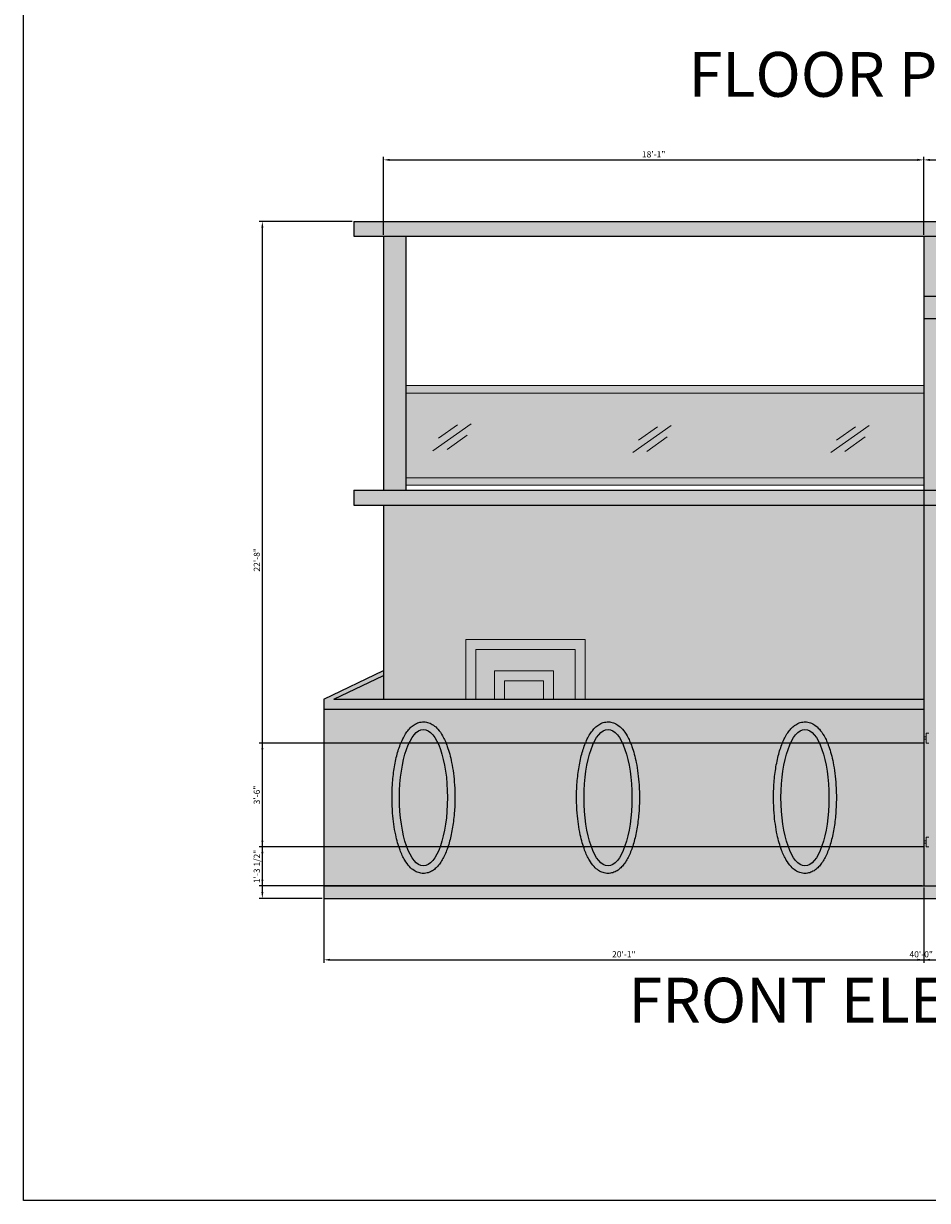
# Model space of a CAD drawing. Units: inches. Extents: x 2169 to 10664, y 1669 to 6352.
# Tile 13 of 17: x 9415 to 9778, y 5159 to 5632. Entities that reach past the tile are written whole.
import ezdxf

# ---------------------------------------------------------------- set-up
doc = ezdxf.new("R2010")
doc.units = ezdxf.units.IN
for name, color, linetype, lineweight in [('A-ANNO-DIMS', 3, 'Continuous', 18), ('A-ANNO-TITL', 3, 'Continuous', 25), ('A-ANNO-TTLB', 7, 'Continuous', 25), ('A-ELEV', 7, 'Continuous', 25), ('A-ELEV-CONC-PATT', 85, 'Continuous', 13), ('A-ELEV-GATE', 7, 'Continuous', 18), ('A-ELEV-GATE-PATT', 252, 'Continuous', 13), ('A-ELEV-OPEN', 7, 'Continuous', 18), ('A-ELEV-OPEN-PATT', 9, 'Continuous', 13), ('A-ELEV-PATT', 253, 'Continuous', 13)]:
    doc.layers.add(name, color=color, linetype=linetype, lineweight=lineweight)
doc.styles.get("Standard").update_dxf_attribs({"font": 'arial.ttf'})
doc.dimstyles.new('ISO-25', dxfattribs={"dimtxt": 2.5, "dimasz": 2.5, "dimexe": 1.25, "dimexo": 0.625, "dimtad": 1, "dimdec": 0, "dimlunit": 3, "dimtxsty": 'Standard', "dimcen": 2.5, "dimadec": 0, "dimazin": 0, "dimtfac": 1, "dimtdec": 0, "dimtmove": 0, "dimatfit": 3, "dimfxl": 1, "dimarcsym": 0})

# ---------------------------------------------------------------- blocks, each defined once
blk = doc.blocks.new('GLASS-MARK-B')
for p, q in [((0, 0), (15.39, 10.84)), ((2.27, 5.02), (9.88, 10.35)), ((5.67, 0.49), (13.77, 6.31))]:
    blk.add_line(p, q)
blk = doc.blocks.new('GATE-HINGE-3')
for p, q in [((1, 2.5), (0, 2.5)), ((1, 1.5), (0, 1.5)), ((2, 4), (1, 4)), ((1, 4), (1, 0)), ((2, 0), (1, 0))]:
    blk.add_line(p, q)
blk = doc.blocks.new('FACADE-OVAL-INSET')
blk.add_ellipse((12.63, 30.44), major_axis=(0, -27.44), ratio=0.350877)
blk.add_open_spline([(12.63, 0), (13.28, 0), (13.93, 0.1), (15.16, 0.48), (15.73, 0.75), (16.8, 1.42), (17.29, 1.81), (18.2, 2.68), (18.63, 3.16), (19.86, 4.78), (20.59, 6.05), (21.9, 8.93), (22.47, 10.53), (23.47, 14), (23.89, 15.87), (24.57, 19.81), (24.82, 21.88), (25.3, 27.78), (25.34, 31.73), (24.89, 38.68), (24.51, 41.73), (23.49, 46.87), (22.91, 49.03), (21.66, 52.55), (21.03, 53.98), (19.74, 56.25), (19.12, 57.16), (17.87, 58.57), (17.27, 59.12), (16.05, 59.96), (15.45, 60.28), (14.17, 60.73), (13.48, 60.86), (12.09, 60.9), (11.4, 60.8), (10.08, 60.4), (9.47, 60.11), (8.34, 59.39), (7.83, 58.96), (6.87, 58.01), (6.43, 57.49), (5.17, 55.76), (4.44, 54.41), (3.14, 51.39), (2.57, 49.71), (1.59, 46.07), (1.19, 44.12), (0.55, 40.02), (0.31, 37.87), (-0.08, 31.9), (-0.06, 28), (0.48, 21.2), (0.89, 18.26), (1.95, 13.31), (2.54, 11.23), (3.8, 7.86), (4.43, 6.5), (5.71, 4.33), (6.34, 3.47), (7.58, 2.13), (8.18, 1.61), (9.39, 0.82), (9.99, 0.52), (11.27, 0.11), (11.95, 0), (12.63, 0)], degree=3, knots=[0, 0, 0, 0, 0.107478, 0.107478, 0.214955, 0.214955, 0.322433, 0.322433, 0.429911, 0.429911, 0.658113, 0.658113, 0.886316, 0.886316, 1.114519, 1.114519, 1.342721, 1.342721, 1.750863, 1.750863, 2.0857, 2.0857, 2.362812, 2.362812, 2.586848, 2.586848, 2.764909, 2.764909, 2.903641, 2.903641, 3.018249, 3.018249, 3.132858, 3.132858, 3.247466, 3.247466, 3.362074, 3.362074, 3.476683, 3.476683, 3.591291, 3.591291, 3.82536, 3.82536, 4.059428, 4.059428, 4.293497, 4.293497, 4.527566, 4.527566, 4.931556, 4.931556, 5.258929, 5.258929, 5.530471, 5.530471, 5.749212, 5.749212, 5.922827, 5.922827, 6.058126, 6.058126, 6.171203, 6.171203, 6.283185, 6.283185, 6.283185, 6.283185])
blk = doc.blocks.new('*D117')
at = {"layer": 'A-ANNO-DIMS', "color": 0, "lineweight": -2, "transparency": 16777216}
for p, q in [((9535.46, 5279.69), (9535.46, 5254.36)), ((10015.46, 5279.69), (10015.46, 5254.36)), ((9537.96, 5255.61), (10012.96, 5255.61))]:
    blk.add_line(p, q, dxfattribs=at)
at = {"layer": 'A-ANNO-DIMS', "color": 0, "transparency": 16777216}
for points in [[(9537.96, 5256.03), (9537.96, 5255.19), (9535.46, 5255.61)], [(10012.96, 5256.03), (10012.96, 5255.19), (10015.46, 5255.61)]]:
    blk.add_solid(points, dxfattribs=at)
at = {"layer": 'Defpoints', "color": 0, "transparency": 16777216}
for p in [(9535.46, 5280.31), (10015.46, 5280.31), (10015.46, 5255.61)]:
    blk.add_point(p, dxfattribs=at)
at = {"layer": 'A-ANNO-DIMS', "color": 0, "transparency": 16777216, "insert": (9775.46, 5257.51), "char_height": 2.5, "attachment_point": 5}
blk.add_mtext('40\'-0"', dxfattribs=at)
blk = doc.blocks.new('*D118')
at = {"layer": 'A-ANNO-DIMS', "color": 0, "lineweight": -2, "transparency": 16777216}
for p, q in [((9546.84, 5552.31), (9509.51, 5552.31)), ((9510.76, 5282.81), (9510.76, 5549.81)), ((9534.84, 5280.31), (9509.51, 5280.31))]:
    blk.add_line(p, q, dxfattribs=at)
at = {"layer": 'A-ANNO-DIMS', "color": 0, "transparency": 16777216}
for points in [[(9510.35, 5549.81), (9511.18, 5549.81), (9510.76, 5552.31)], [(9510.35, 5282.81), (9511.18, 5282.81), (9510.76, 5280.31)]]:
    blk.add_solid(points, dxfattribs=at)
at = {"layer": 'Defpoints', "color": 0, "transparency": 16777216}
for p in [(9510.76, 5552.31), (9547.46, 5552.31), (9535.46, 5280.31)]:
    blk.add_point(p, dxfattribs=at)
at = {"layer": 'A-ANNO-DIMS', "color": 0, "transparency": 16777216, "insert": (9508.86, 5416.31), "char_height": 2.5, "attachment_point": 5, "rotation": 90}
blk.add_mtext('22\'-8"', dxfattribs=at)
blk = doc.blocks.new('*D120')
at = {"layer": 'A-ANNO-DIMS', "color": 0, "lineweight": -2, "transparency": 16777216}
for p, q in [((9535.46, 5284.69), (9535.46, 5254.36)), ((9776.46, 5284.69), (9776.46, 5254.36)), ((9537.96, 5255.61), (9773.96, 5255.61))]:
    blk.add_line(p, q, dxfattribs=at)
at = {"layer": 'A-ANNO-DIMS', "color": 0, "transparency": 16777216}
for points in [[(9537.96, 5256.03), (9537.96, 5255.19), (9535.46, 5255.61)], [(9773.96, 5256.03), (9773.96, 5255.19), (9776.46, 5255.61)]]:
    blk.add_solid(points, dxfattribs=at)
at = {"layer": 'Defpoints', "color": 0, "transparency": 16777216}
for p in [(9535.46, 5285.31), (9776.46, 5285.31), (9776.46, 5255.61)]:
    blk.add_point(p, dxfattribs=at)
at = {"layer": 'A-ANNO-DIMS', "color": 0, "transparency": 16777216, "insert": (9655.96, 5257.51), "char_height": 2.5, "attachment_point": 5}
blk.add_mtext('20\'-1"', dxfattribs=at)
blk = doc.blocks.new('*D121')
at = {"layer": 'A-ANNO-DIMS', "color": 0, "lineweight": -2, "transparency": 16777216}
for p, q in [((9559.46, 5546.94), (9559.46, 5578.26)), ((9561.96, 5577.01), (9773.96, 5577.01)), ((9776.46, 5546.94), (9776.46, 5578.26))]:
    blk.add_line(p, q, dxfattribs=at)
at = {"layer": 'A-ANNO-DIMS', "color": 0, "transparency": 16777216}
for points in [[(9561.96, 5577.43), (9561.96, 5576.59), (9559.46, 5577.01)], [(9773.96, 5577.43), (9773.96, 5576.59), (9776.46, 5577.01)]]:
    blk.add_solid(points, dxfattribs=at)
at = {"layer": 'Defpoints', "color": 0, "transparency": 16777216}
for p in [(9776.46, 5577.01), (9559.46, 5546.31), (9776.46, 5546.31)]:
    blk.add_point(p, dxfattribs=at)
at = {"layer": 'A-ANNO-DIMS', "color": 0, "transparency": 16777216, "insert": (9667.96, 5578.91), "char_height": 2.5, "attachment_point": 5}
blk.add_mtext('18\'-1"', dxfattribs=at)
blk = doc.blocks.new('*D122')
at = {"layer": 'A-ANNO-DIMS', "color": 0, "lineweight": -2, "transparency": 16777216}
for p, q in [((9776.46, 5546.94), (9776.46, 5578.26)), ((9778.96, 5577.01), (9932.96, 5577.01)), ((9935.46, 5546.94), (9935.46, 5578.26))]:
    blk.add_line(p, q, dxfattribs=at)
at = {"layer": 'A-ANNO-DIMS', "color": 0, "transparency": 16777216}
for points in [[(9778.96, 5577.43), (9778.96, 5576.59), (9776.46, 5577.01)], [(9932.96, 5577.43), (9932.96, 5576.59), (9935.46, 5577.01)]]:
    blk.add_solid(points, dxfattribs=at)
at = {"layer": 'Defpoints', "color": 0, "transparency": 16777216}
for p in [(9935.46, 5577.01), (9776.46, 5546.31), (9935.46, 5546.31)]:
    blk.add_point(p, dxfattribs=at)
at = {"layer": 'A-ANNO-DIMS', "color": 0, "transparency": 16777216, "insert": (9855.96, 5578.91), "char_height": 2.5, "attachment_point": 5}
blk.add_mtext('13\'-3"', dxfattribs=at)
blk = doc.blocks.new('*D124')
at = {"layer": 'A-ANNO-DIMS', "color": 0, "lineweight": -2, "transparency": 16777216}
for p, q in [((9776.46, 5284.69), (9776.46, 5254.36)), ((9848.46, 5284.69), (9848.46, 5254.36)), ((9778.96, 5255.61), (9845.96, 5255.61))]:
    blk.add_line(p, q, dxfattribs=at)
at = {"layer": 'A-ANNO-DIMS', "color": 0, "transparency": 16777216}
for points in [[(9778.96, 5256.03), (9778.96, 5255.19), (9776.46, 5255.61)], [(9845.96, 5256.03), (9845.96, 5255.19), (9848.46, 5255.61)]]:
    blk.add_solid(points, dxfattribs=at)
at = {"layer": 'Defpoints', "color": 0, "transparency": 16777216}
for p in [(9776.46, 5285.31), (9848.46, 5285.31), (9848.46, 5255.61)]:
    blk.add_point(p, dxfattribs=at)
at = {"layer": 'A-ANNO-DIMS', "color": 0, "transparency": 16777216, "insert": (9812.46, 5257.51), "char_height": 2.5, "attachment_point": 5}
blk.add_mtext('6\'-0"', dxfattribs=at)
blk = doc.blocks.new('*D126')
at = {"layer": 'A-ANNO-DIMS', "color": 0, "lineweight": -2, "transparency": 16777216}
for p, q in [((9776.84, 5300.95), (9509.51, 5300.95)), ((9510.76, 5287.81), (9510.76, 5298.45)), ((9775.84, 5285.31), (9509.51, 5285.31))]:
    blk.add_line(p, q, dxfattribs=at)
at = {"layer": 'A-ANNO-DIMS', "color": 0, "transparency": 16777216}
for points in [[(9510.35, 5298.45), (9511.18, 5298.45), (9510.76, 5300.95)], [(9510.35, 5287.81), (9511.18, 5287.81), (9510.76, 5285.31)]]:
    blk.add_solid(points, dxfattribs=at)
at = {"layer": 'Defpoints', "color": 0, "transparency": 16777216}
for p in [(9510.76, 5300.95), (9777.46, 5300.95), (9776.46, 5285.31)]:
    blk.add_point(p, dxfattribs=at)
at = {"layer": 'A-ANNO-DIMS', "color": 0, "transparency": 16777216, "insert": (9508.84, 5293.13), "char_height": 2.5, "attachment_point": 5, "rotation": 90}
blk.add_mtext('1\'-3 1/2"', dxfattribs=at)
blk = doc.blocks.new('*D127')
at = {"layer": 'A-ANNO-DIMS', "color": 0, "lineweight": -2, "transparency": 16777216}
for p, q in [((9776.84, 5342.71), (9509.51, 5342.71)), ((9510.76, 5303.45), (9510.76, 5340.21)), ((9776.84, 5300.95), (9509.51, 5300.95))]:
    blk.add_line(p, q, dxfattribs=at)
at = {"layer": 'A-ANNO-DIMS', "color": 0, "transparency": 16777216}
for points in [[(9510.35, 5340.21), (9511.18, 5340.21), (9510.76, 5342.71)], [(9510.35, 5303.45), (9511.18, 5303.45), (9510.76, 5300.95)]]:
    blk.add_solid(points, dxfattribs=at)
at = {"layer": 'Defpoints', "color": 0, "transparency": 16777216}
for p in [(9510.76, 5342.71), (9777.46, 5342.71), (9777.46, 5300.95)]:
    blk.add_point(p, dxfattribs=at)
at = {"layer": 'A-ANNO-DIMS', "color": 0, "transparency": 16777216, "insert": (9508.86, 5321.83), "char_height": 2.5, "attachment_point": 5, "rotation": 90}
blk.add_mtext('3\'-6"', dxfattribs=at)

msp = doc.modelspace()

# ---------------------------------------------------------------- hatches: boundary and pattern name
at = {"layer": 'A-ELEV-CONC-PATT'}
h = msp.add_hatch(dxfattribs=at)
h.set_pattern_fill('AR-CONC', color=256, scale=0.02)
h.paths.add_polyline_path([(9899.46, 5522.31), (9776.46, 5522.31), (9776.46, 5513.31), (9890.46, 5513.31), (9890.46, 5444.31), (9899.46, 5444.31)])
h.paths.add_polyline_path([(9899.46, 5438.31), (9890.46, 5438.31), (9890.46, 5285.31), (9899.46, 5285.31)])
at = {"layer": 'A-ELEV-GATE-PATT'}
h = msp.add_hatch(color=256, dxfattribs=at)
h.dxf.hatch_style = 1
h.paths.add_polyline_path([(9778.46, 5346.71), (9777.46, 5346.71), (9777.46, 5342.71), (9778.46, 5342.71)])
h.paths.add_polyline_path([(9777.46, 5345.21), (9776.46, 5345.21), (9776.46, 5344.21), (9777.46, 5344.21)])
h.paths.add_polyline_path([(9848.46, 5345.21), (9847.46, 5345.21), (9847.46, 5344.21), (9848.46, 5344.21)])
h.paths.add_polyline_path([(9847.46, 5346.71), (9846.46, 5346.71), (9846.46, 5342.71), (9847.46, 5342.71)])
h.paths.add_polyline_path([(9847.46, 5304.95), (9846.46, 5304.95), (9846.46, 5300.95), (9847.46, 5300.95)])
h.paths.add_polyline_path([(9848.46, 5303.45), (9847.46, 5303.45), (9847.46, 5302.45), (9848.46, 5302.45)])
h.paths.add_polyline_path([(9778.46, 5304.95), (9777.46, 5304.95), (9777.46, 5300.95), (9778.46, 5300.95)])
h.paths.add_polyline_path([(9777.46, 5303.45), (9776.46, 5303.45), (9776.46, 5302.45), (9777.46, 5302.45)])
h.paths.add_polyline_path([(9811.96, 5360.31), (9778.46, 5360.31), (9778.46, 5287.31), (9811.96, 5287.31)])
h.paths.add_polyline_path([(9783.46, 5355.31), (9806.96, 5355.31), (9806.96, 5292.31), (9783.46, 5292.31)], flags=16)
h.paths.add_polyline_path([(9788.71, 5349.82), (9801.33, 5349.82), (9801.33, 5298.27), (9788.71, 5298.27)], flags=0)
h.paths.add_polyline_path([(9791.71, 5346.82), (9798.33, 5346.82), (9798.33, 5301.27), (9791.71, 5301.27)], flags=0)
h.paths.add_polyline_path([(9807.16, 5332.61, -1), (9811.54, 5332.61, -1)], flags=16)
h.paths.add_polyline_path([(9808.16, 5332.61, -1), (9810.54, 5332.61, -1)], flags=0)
h.paths.add_polyline_path([(9846.46, 5360.31), (9812.96, 5360.31), (9812.96, 5287.31), (9846.46, 5287.31)])
h.paths.add_polyline_path([(9817.96, 5355.31), (9841.46, 5355.31), (9841.46, 5292.31), (9817.96, 5292.31)], flags=16)
h.paths.add_polyline_path([(9823.29, 5349.82), (9835.91, 5349.82), (9835.91, 5298.27), (9823.29, 5298.27)], flags=0)
h.paths.add_polyline_path([(9826.29, 5346.82), (9832.91, 5346.82), (9832.91, 5301.27), (9826.29, 5301.27)], flags=0)
h.paths.add_polyline_path([(9813.3, 5332.61, -1), (9817.67, 5332.61, -1)], flags=16)
h.paths.add_polyline_path([(9814.3, 5332.61, -1), (9816.67, 5332.61, -1)], flags=0)
h.paths.add_polyline_path([(9801.33, 5349.82), (9788.71, 5349.82), (9788.71, 5298.27), (9801.33, 5298.27)], flags=0)
at = {"layer": 'A-ELEV-OPEN-PATT'}
h = msp.add_hatch(color=256, dxfattribs=at)
h.dxf.hatch_style = 1
h.paths.add_polyline_path([(9776.46, 5449.31), (9568.46, 5449.31), (9568.46, 5446.31), (9776.46, 5446.31)])
h.paths.add_polyline_path([(9776.46, 5486.31), (9568.46, 5486.31), (9568.46, 5483.31), (9776.46, 5483.31)])
h = msp.add_hatch(color=256, dxfattribs=at)
h.dxf.hatch_style = 1
h.paths.add_polyline_path([(9776.46, 5483.31), (9568.46, 5483.31), (9568.46, 5449.31), (9776.46, 5449.31)])
h = msp.add_hatch(color=256, dxfattribs=at)
h.dxf.hatch_style = 1
h.paths.add_polyline_path([(9836.46, 5384.31), (9788.46, 5384.31), (9788.46, 5360.31), (9792.46, 5360.31), (9792.46, 5380.31), (9832.46, 5380.31), (9832.46, 5360.31), (9836.46, 5360.31)])
h.paths.add_polyline_path([(9823.12, 5371.65), (9801.1, 5371.65), (9801.1, 5360.31), (9805.1, 5360.31), (9805.1, 5367.65), (9819.12, 5367.65), (9819.12, 5360.31), (9823.12, 5360.31)], flags=17)
h.paths.add_polyline_path([(9640.46, 5384.31), (9592.46, 5384.31), (9592.46, 5360.31), (9596.46, 5360.31), (9596.46, 5380.31), (9636.46, 5380.31), (9636.46, 5360.31), (9640.46, 5360.31)])
h.paths.add_polyline_path([(9627.69, 5371.73), (9604, 5371.73), (9604, 5360.31), (9608, 5360.31), (9608, 5367.73), (9623.69, 5367.73), (9623.69, 5360.31), (9627.69, 5360.31)], flags=17)
h = msp.add_hatch(color=256, dxfattribs=at)
h.dxf.hatch_style = 1
h.paths.add_polyline_path([(9636.46, 5380.31), (9596.46, 5380.31), (9596.46, 5360.31), (9604, 5360.31), (9604, 5371.73), (9627.69, 5371.73), (9627.69, 5360.31), (9636.46, 5360.31)])
h.paths.add_polyline_path([(9623.69, 5367.73), (9608, 5367.73), (9608, 5360.31), (9623.69, 5360.31)], flags=17)
h.paths.add_polyline_path([(9832.46, 5380.31), (9792.46, 5380.31), (9792.46, 5360.31), (9801.1, 5360.31), (9801.1, 5371.65), (9823.12, 5371.65), (9823.12, 5360.31), (9832.46, 5360.31)])
at = {"layer": 'A-ELEV-PATT'}
h = msp.add_hatch(color=256, dxfattribs=at)
h.dxf.hatch_style = 1
h.paths.add_polyline_path([(10003.46, 5552.31), (9547.46, 5552.31), (9547.46, 5546.31), (10003.46, 5546.31)])
h.paths.add_polyline_path([(9776.46, 5444.31), (9547.46, 5444.31), (9547.46, 5438.31), (9776.46, 5438.31)])
h.paths.add_polyline_path([(9935.46, 5444.31), (9776.46, 5444.31), (9776.46, 5438.31), (9935.46, 5438.31)])
h.paths.add_polyline_path([(10003.46, 5444.31), (9935.46, 5444.31), (9935.46, 5438.31), (10003.46, 5438.31)])
h = msp.add_hatch(color=256, dxfattribs=at)
h.dxf.hatch_style = 1
h.paths.add_polyline_path([(9568.46, 5546.31), (9559.46, 5546.31), (9559.46, 5444.31), (9568.46, 5444.31)])
h = msp.add_hatch(color=256, dxfattribs=at)
h.dxf.hatch_style = 1
h.paths.add_polyline_path([(9935.46, 5546.31), (9776.46, 5546.31), (9776.46, 5522.31), (9899.46, 5522.31), (9899.46, 5444.31), (9935.46, 5444.31)])
h.paths.add_polyline_path([(9935.46, 5438.31), (9899.46, 5438.31), (9899.46, 5285.31), (9935.46, 5285.31)])
h.paths.add_polyline_path([(9890.46, 5438.31), (9848.46, 5438.31), (9848.46, 5285.31), (9890.46, 5285.31)])
h.paths.add_polyline_path([(9890.46, 5513.31), (9776.46, 5513.31), (9776.46, 5444.31), (9890.46, 5444.31)], flags=17)
h = msp.add_hatch(color=256, dxfattribs=at)
h.dxf.hatch_style = 1
h.paths.add_polyline_path([(9776.46, 5438.31), (9559.46, 5438.31), (9559.46, 5360.31), (9592.46, 5360.31), (9592.46, 5384.31), (9640.46, 5384.31), (9640.46, 5360.31), (9776.46, 5360.31)])
h = msp.add_hatch(color=256, dxfattribs=at)
h.dxf.hatch_style = 1
h.paths.add_polyline_path([(9848.46, 5438.31), (9776.46, 5438.31), (9776.46, 5345.21), (9777.46, 5345.21), (9777.46, 5346.71), (9778.46, 5346.71), (9778.46, 5360.31), (9788.46, 5360.31), (9788.46, 5384.31), (9836.46, 5384.31), (9836.46, 5360.31), (9846.46, 5360.31), (9846.46, 5346.71), (9847.46, 5346.71), (9847.46, 5345.21), (9848.46, 5345.21)])
h = msp.add_hatch(color=256, dxfattribs=at)
h.dxf.hatch_style = 1
h.paths.add_polyline_path([(9776.46, 5360.31), (9539.46, 5360.31), (9559.46, 5369.86), (9559.46, 5371.85), (9535.46, 5360.31), (9535.46, 5356.31), (9776.46, 5356.31)])
h.paths.add_polyline_path([(10015.46, 5360.31), (9991.46, 5372.52), (9991.46, 5370.33), (10011.46, 5360.31), (9935.46, 5360.31), (9935.46, 5356.31), (10015.46, 5356.31)])
h = msp.add_hatch(color=256, dxfattribs=at)
h.dxf.hatch_style = 1
h.paths.add_polyline_path([(9559.46, 5369.86), (9539.46, 5360.31), (9559.46, 5360.31)])
h.paths.add_polyline_path([(9991.46, 5370.33), (9991.46, 5360.31), (10011.46, 5360.31)])
h = msp.add_hatch(color=256, dxfattribs=at)
h.dxf.hatch_style = 1
h.paths.add_polyline_path([(9778.46, 5342.71), (9777.46, 5342.71), (9777.46, 5344.21), (9776.46, 5344.21), (9776.46, 5303.45), (9777.46, 5303.45), (9777.46, 5304.95), (9778.46, 5304.95)], flags=17)
h.paths.add_polyline_path([(9848.46, 5344.21), (9847.46, 5344.21), (9847.46, 5342.71), (9846.46, 5342.71), (9846.46, 5304.95), (9847.46, 5304.95), (9847.46, 5303.45), (9848.46, 5303.45)], flags=17)
h.paths.add_polyline_path([(9778.46, 5300.95), (9777.46, 5300.95), (9777.46, 5302.45), (9776.46, 5302.45), (9776.46, 5285.31), (9848.46, 5285.31), (9848.46, 5302.45), (9847.46, 5302.45), (9847.46, 5300.95), (9846.46, 5300.95), (9846.46, 5287.31), (9812.96, 5287.31), (9812.96, 5360.31), (9819.12, 5360.31), (9819.12, 5367.65), (9805.1, 5367.65), (9805.1, 5360.31), (9811.96, 5360.31), (9811.96, 5287.31), (9778.46, 5287.31)])
h = msp.add_hatch(color=256, dxfattribs=at)
h.dxf.hatch_style = 1
h.paths.add_polyline_path([(9776.46, 5356.31), (9535.46, 5356.31), (9535.46, 5285.31), (9776.46, 5285.31)])
edge = h.paths.add_edge_path(flags=16)
edge.add_spline(control_points=[(9649.63, 5290.33), (9650.28, 5290.33), (9650.93, 5290.43), (9652.16, 5290.81), (9652.74, 5291.08), (9653.8, 5291.75), (9654.29, 5292.14), (9655.21, 5293.01), (9655.63, 5293.48), (9656.87, 5295.1), (9657.6, 5296.38), (9658.9, 5299.26), (9659.48, 5300.86), (9660.47, 5304.33), (9660.89, 5306.2), (9661.57, 5310.14), (9661.83, 5312.21), (9662.31, 5318.11), (9662.34, 5322.06), (9661.9, 5329.01), (9661.51, 5332.06), (9660.49, 5337.2), (9659.91, 5339.36), (9658.66, 5342.88), (9658.03, 5344.31), (9656.74, 5346.58), (9656.12, 5347.49), (9654.87, 5348.9), (9654.27, 5349.45), (9653.06, 5350.29), (9652.46, 5350.61), (9651.17, 5351.06), (9650.48, 5351.19), (9649.1, 5351.23), (9648.4, 5351.13), (9647.09, 5350.73), (9646.47, 5350.44), (9645.35, 5349.72), (9644.83, 5349.29), (9643.87, 5348.34), (9643.43, 5347.82), (9642.18, 5346.09), (9641.44, 5344.74), (9640.14, 5341.72), (9639.57, 5340.04), (9638.6, 5336.4), (9638.19, 5334.45), (9637.55, 5330.34), (9637.32, 5328.2), (9636.93, 5322.23), (9636.95, 5318.33), (9637.48, 5311.53), (9637.89, 5308.59), (9638.95, 5303.64), (9639.54, 5301.56), (9640.8, 5298.19), (9641.43, 5296.83), (9642.72, 5294.66), (9643.34, 5293.8), (9644.59, 5292.46), (9645.18, 5291.94), (9646.4, 5291.15), (9647, 5290.85), (9648.28, 5290.44), (9648.95, 5290.33), (9649.63, 5290.33)], knot_values=[0, 0, 0, 0, 0.107478, 0.107478, 0.214955, 0.214955, 0.322433, 0.322433, 0.429911, 0.429911, 0.658113, 0.658113, 0.886316, 0.886316, 1.114519, 1.114519, 1.342721, 1.342721, 1.750863, 1.750863, 2.0857, 2.0857, 2.362812, 2.362812, 2.586848, 2.586848, 2.764909, 2.764909, 2.903641, 2.903641, 3.018249, 3.018249, 3.132858, 3.132858, 3.247466, 3.247466, 3.362074, 3.362074, 3.476683, 3.476683, 3.591291, 3.591291, 3.82536, 3.82536, 4.059428, 4.059428, 4.293497, 4.293497, 4.527566, 4.527566, 4.931556, 4.931556, 5.258929, 5.258929, 5.530471, 5.530471, 5.749212, 5.749212, 5.922827, 5.922827, 6.058126, 6.058126, 6.171203, 6.171203, 6.283185, 6.283185, 6.283185, 6.283185], degree=3, periodic=0)
edge = h.paths.add_edge_path(flags=16)
edge.add_spline(control_points=[(9575.48, 5290.33), (9576.13, 5290.33), (9576.78, 5290.43), (9578.01, 5290.81), (9578.59, 5291.08), (9579.65, 5291.75), (9580.15, 5292.14), (9581.06, 5293.01), (9581.48, 5293.48), (9582.72, 5295.1), (9583.45, 5296.38), (9584.76, 5299.26), (9585.33, 5300.86), (9586.32, 5304.33), (9586.74, 5306.2), (9587.42, 5310.14), (9587.68, 5312.21), (9588.16, 5318.11), (9588.19, 5322.06), (9587.75, 5329.01), (9587.36, 5332.06), (9586.34, 5337.2), (9585.76, 5339.36), (9584.51, 5342.88), (9583.88, 5344.31), (9582.59, 5346.58), (9581.97, 5347.49), (9580.72, 5348.9), (9580.12, 5349.45), (9578.91, 5350.29), (9578.31, 5350.61), (9577.02, 5351.06), (9576.33, 5351.19), (9574.95, 5351.23), (9574.25, 5351.13), (9572.94, 5350.73), (9572.33, 5350.44), (9571.2, 5349.72), (9570.68, 5349.29), (9569.72, 5348.34), (9569.28, 5347.82), (9568.03, 5346.09), (9567.29, 5344.74), (9565.99, 5341.72), (9565.42, 5340.04), (9564.45, 5336.4), (9564.04, 5334.45), (9563.4, 5330.34), (9563.17, 5328.2), (9562.78, 5322.23), (9562.8, 5318.33), (9563.33, 5311.53), (9563.74, 5308.59), (9564.8, 5303.64), (9565.39, 5301.56), (9566.65, 5298.19), (9567.29, 5296.83), (9568.57, 5294.66), (9569.19, 5293.8), (9570.44, 5292.46), (9571.03, 5291.94), (9572.25, 5291.15), (9572.85, 5290.85), (9574.13, 5290.44), (9574.8, 5290.33), (9575.48, 5290.33)], knot_values=[0, 0, 0, 0, 0.107478, 0.107478, 0.214955, 0.214955, 0.322433, 0.322433, 0.429911, 0.429911, 0.658113, 0.658113, 0.886316, 0.886316, 1.114519, 1.114519, 1.342721, 1.342721, 1.750863, 1.750863, 2.0857, 2.0857, 2.362812, 2.362812, 2.586848, 2.586848, 2.764909, 2.764909, 2.903641, 2.903641, 3.018249, 3.018249, 3.132858, 3.132858, 3.247466, 3.247466, 3.362074, 3.362074, 3.476683, 3.476683, 3.591291, 3.591291, 3.82536, 3.82536, 4.059428, 4.059428, 4.293497, 4.293497, 4.527566, 4.527566, 4.931556, 4.931556, 5.258929, 5.258929, 5.530471, 5.530471, 5.749212, 5.749212, 5.922827, 5.922827, 6.058126, 6.058126, 6.171203, 6.171203, 6.283185, 6.283185, 6.283185, 6.283185], degree=3, periodic=0)
edge = h.paths.add_edge_path(flags=0)
edge.add_ellipse((9649.63, 5320.77), major_axis=(0, -27.44), ratio=0.350877, start_angle=0, end_angle=360)
edge = h.paths.add_edge_path(flags=0)
edge.add_ellipse((9575.48, 5320.77), major_axis=(0, -27.44), ratio=0.350877, start_angle=0, end_angle=360)
edge = h.paths.add_edge_path(flags=16)
edge.add_spline(control_points=[(9728.75, 5290.33), (9729.4, 5290.33), (9730.05, 5290.43), (9731.28, 5290.81), (9731.86, 5291.08), (9732.92, 5291.75), (9733.41, 5292.14), (9734.33, 5293.01), (9734.75, 5293.48), (9735.99, 5295.1), (9736.72, 5296.38), (9738.02, 5299.26), (9738.6, 5300.86), (9739.59, 5304.33), (9740.01, 5306.2), (9740.69, 5310.14), (9740.95, 5312.21), (9741.43, 5318.11), (9741.46, 5322.06), (9741.02, 5329.01), (9740.63, 5332.06), (9739.61, 5337.2), (9739.03, 5339.36), (9737.78, 5342.88), (9737.15, 5344.31), (9735.86, 5346.58), (9735.24, 5347.49), (9733.99, 5348.9), (9733.39, 5349.45), (9732.18, 5350.29), (9731.58, 5350.61), (9730.29, 5351.06), (9729.6, 5351.19), (9728.22, 5351.23), (9727.52, 5351.13), (9726.21, 5350.73), (9725.59, 5350.44), (9724.47, 5349.72), (9723.95, 5349.29), (9722.99, 5348.34), (9722.55, 5347.82), (9721.29, 5346.09), (9720.56, 5344.74), (9719.26, 5341.72), (9718.69, 5340.04), (9717.72, 5336.4), (9717.31, 5334.45), (9716.67, 5330.34), (9716.44, 5328.2), (9716.04, 5322.23), (9716.07, 5318.33), (9716.6, 5311.53), (9717.01, 5308.59), (9718.07, 5303.64), (9718.66, 5301.56), (9719.92, 5298.19), (9720.55, 5296.83), (9721.84, 5294.66), (9722.46, 5293.8), (9723.71, 5292.46), (9724.3, 5291.94), (9725.52, 5291.15), (9726.12, 5290.85), (9727.4, 5290.44), (9728.07, 5290.33), (9728.75, 5290.33)], knot_values=[0, 0, 0, 0, 0.107478, 0.107478, 0.214955, 0.214955, 0.322433, 0.322433, 0.429911, 0.429911, 0.658113, 0.658113, 0.886316, 0.886316, 1.114519, 1.114519, 1.342721, 1.342721, 1.750863, 1.750863, 2.0857, 2.0857, 2.362812, 2.362812, 2.586848, 2.586848, 2.764909, 2.764909, 2.903641, 2.903641, 3.018249, 3.018249, 3.132858, 3.132858, 3.247466, 3.247466, 3.362074, 3.362074, 3.476683, 3.476683, 3.591291, 3.591291, 3.82536, 3.82536, 4.059428, 4.059428, 4.293497, 4.293497, 4.527566, 4.527566, 4.931556, 4.931556, 5.258929, 5.258929, 5.530471, 5.530471, 5.749212, 5.749212, 5.922827, 5.922827, 6.058126, 6.058126, 6.171203, 6.171203, 6.283185, 6.283185, 6.283185, 6.283185], degree=3, periodic=0)
edge = h.paths.add_edge_path(flags=0)
edge.add_ellipse((9728.75, 5320.77), major_axis=(0, -27.44), ratio=0.350877, start_angle=0, end_angle=360)
h.paths.add_polyline_path([(10015.46, 5356.31), (9935.46, 5356.31), (9935.46, 5285.31), (10015.46, 5285.31)])
edge = h.paths.add_edge_path(flags=16)
edge.add_spline(control_points=[(9976.67, 5290.33), (9977.32, 5290.33), (9977.97, 5290.43), (9979.2, 5290.81), (9979.78, 5291.08), (9980.85, 5291.75), (9981.34, 5292.14), (9982.25, 5293.01), (9982.67, 5293.48), (9983.91, 5295.1), (9984.64, 5296.38), (9985.95, 5299.26), (9986.52, 5300.86), (9987.51, 5304.33), (9987.93, 5306.2), (9988.61, 5310.14), (9988.87, 5312.21), (9989.35, 5318.11), (9989.38, 5322.06), (9988.94, 5329.01), (9988.55, 5332.06), (9987.53, 5337.2), (9986.95, 5339.36), (9985.7, 5342.88), (9985.07, 5344.31), (9983.79, 5346.58), (9983.16, 5347.49), (9981.91, 5348.9), (9981.31, 5349.45), (9980.1, 5350.29), (9979.5, 5350.61), (9978.21, 5351.06), (9977.53, 5351.19), (9976.14, 5351.23), (9975.44, 5351.13), (9974.13, 5350.73), (9973.52, 5350.44), (9972.39, 5349.72), (9971.87, 5349.29), (9970.91, 5348.34), (9970.47, 5347.82), (9969.22, 5346.09), (9968.49, 5344.74), (9967.18, 5341.72), (9966.62, 5340.04), (9965.64, 5336.4), (9965.23, 5334.45), (9964.59, 5330.34), (9964.36, 5328.2), (9963.97, 5322.23), (9963.99, 5318.33), (9964.52, 5311.53), (9964.94, 5308.59), (9965.99, 5303.64), (9966.58, 5301.56), (9967.84, 5298.19), (9968.48, 5296.83), (9969.76, 5294.66), (9970.38, 5293.8), (9971.63, 5292.46), (9972.22, 5291.94), (9973.44, 5291.15), (9974.04, 5290.85), (9975.32, 5290.44), (9975.99, 5290.33), (9976.67, 5290.33)], knot_values=[0, 0, 0, 0, 0.107478, 0.107478, 0.214955, 0.214955, 0.322433, 0.322433, 0.429911, 0.429911, 0.658113, 0.658113, 0.886316, 0.886316, 1.114519, 1.114519, 1.342721, 1.342721, 1.750863, 1.750863, 2.0857, 2.0857, 2.362812, 2.362812, 2.586848, 2.586848, 2.764909, 2.764909, 2.903641, 2.903641, 3.018249, 3.018249, 3.132858, 3.132858, 3.247466, 3.247466, 3.362074, 3.362074, 3.476683, 3.476683, 3.591291, 3.591291, 3.82536, 3.82536, 4.059428, 4.059428, 4.293497, 4.293497, 4.527566, 4.527566, 4.931556, 4.931556, 5.258929, 5.258929, 5.530471, 5.530471, 5.749212, 5.749212, 5.922827, 5.922827, 6.058126, 6.058126, 6.171203, 6.171203, 6.283185, 6.283185, 6.283185, 6.283185], degree=3, periodic=0)
edge = h.paths.add_edge_path(flags=0)
edge.add_ellipse((9976.67, 5320.77), major_axis=(0, -27.44), ratio=0.350877, start_angle=0, end_angle=360)
h = msp.add_hatch(color=256, dxfattribs=at)
h.dxf.hatch_style = 1
edge = h.paths.add_edge_path()
edge.add_spline(control_points=[(9575.48, 5290.33), (9576.13, 5290.33), (9576.78, 5290.43), (9578.01, 5290.81), (9578.59, 5291.08), (9579.65, 5291.75), (9580.15, 5292.14), (9581.06, 5293.01), (9581.48, 5293.48), (9582.72, 5295.1), (9583.45, 5296.38), (9584.76, 5299.26), (9585.33, 5300.86), (9586.32, 5304.33), (9586.74, 5306.2), (9587.42, 5310.14), (9587.68, 5312.21), (9588.16, 5318.11), (9588.19, 5322.06), (9587.75, 5329.01), (9587.36, 5332.06), (9586.34, 5337.2), (9585.76, 5339.36), (9584.51, 5342.88), (9583.88, 5344.31), (9582.59, 5346.58), (9581.97, 5347.49), (9580.72, 5348.9), (9580.12, 5349.45), (9578.91, 5350.29), (9578.31, 5350.61), (9577.02, 5351.06), (9576.33, 5351.19), (9574.95, 5351.23), (9574.25, 5351.13), (9572.94, 5350.73), (9572.33, 5350.44), (9571.2, 5349.72), (9570.68, 5349.29), (9569.72, 5348.34), (9569.28, 5347.82), (9568.03, 5346.09), (9567.29, 5344.74), (9565.99, 5341.72), (9565.42, 5340.04), (9564.45, 5336.4), (9564.04, 5334.45), (9563.4, 5330.34), (9563.17, 5328.2), (9562.78, 5322.23), (9562.8, 5318.33), (9563.33, 5311.53), (9563.74, 5308.59), (9564.8, 5303.64), (9565.39, 5301.56), (9566.65, 5298.19), (9567.29, 5296.83), (9568.57, 5294.66), (9569.19, 5293.8), (9570.44, 5292.46), (9571.03, 5291.94), (9572.25, 5291.15), (9572.85, 5290.85), (9574.13, 5290.44), (9574.8, 5290.33), (9575.48, 5290.33)], knot_values=[0, 0, 0, 0, 0.107478, 0.107478, 0.214955, 0.214955, 0.322433, 0.322433, 0.429911, 0.429911, 0.658113, 0.658113, 0.886316, 0.886316, 1.114519, 1.114519, 1.342721, 1.342721, 1.750863, 1.750863, 2.0857, 2.0857, 2.362812, 2.362812, 2.586848, 2.586848, 2.764909, 2.764909, 2.903641, 2.903641, 3.018249, 3.018249, 3.132858, 3.132858, 3.247466, 3.247466, 3.362074, 3.362074, 3.476683, 3.476683, 3.591291, 3.591291, 3.82536, 3.82536, 4.059428, 4.059428, 4.293497, 4.293497, 4.527566, 4.527566, 4.931556, 4.931556, 5.258929, 5.258929, 5.530471, 5.530471, 5.749212, 5.749212, 5.922827, 5.922827, 6.058126, 6.058126, 6.171203, 6.171203, 6.283185, 6.283185, 6.283185, 6.283185], degree=3, periodic=0)
edge = h.paths.add_edge_path(flags=16)
edge.add_ellipse((9575.48, 5320.77), major_axis=(0, -27.44), ratio=0.350877, start_angle=0, end_angle=360)
edge = h.paths.add_edge_path()
edge.add_spline(control_points=[(9649.63, 5290.33), (9650.28, 5290.33), (9650.93, 5290.43), (9652.16, 5290.81), (9652.74, 5291.08), (9653.8, 5291.75), (9654.29, 5292.14), (9655.21, 5293.01), (9655.63, 5293.48), (9656.87, 5295.1), (9657.6, 5296.38), (9658.9, 5299.26), (9659.48, 5300.86), (9660.47, 5304.33), (9660.89, 5306.2), (9661.57, 5310.14), (9661.83, 5312.21), (9662.31, 5318.11), (9662.34, 5322.06), (9661.9, 5329.01), (9661.51, 5332.06), (9660.49, 5337.2), (9659.91, 5339.36), (9658.66, 5342.88), (9658.03, 5344.31), (9656.74, 5346.58), (9656.12, 5347.49), (9654.87, 5348.9), (9654.27, 5349.45), (9653.06, 5350.29), (9652.46, 5350.61), (9651.17, 5351.06), (9650.48, 5351.19), (9649.1, 5351.23), (9648.4, 5351.13), (9647.09, 5350.73), (9646.47, 5350.44), (9645.35, 5349.72), (9644.83, 5349.29), (9643.87, 5348.34), (9643.43, 5347.82), (9642.18, 5346.09), (9641.44, 5344.74), (9640.14, 5341.72), (9639.57, 5340.04), (9638.6, 5336.4), (9638.19, 5334.45), (9637.55, 5330.34), (9637.32, 5328.2), (9636.93, 5322.23), (9636.95, 5318.33), (9637.48, 5311.53), (9637.89, 5308.59), (9638.95, 5303.64), (9639.54, 5301.56), (9640.8, 5298.19), (9641.43, 5296.83), (9642.72, 5294.66), (9643.34, 5293.8), (9644.59, 5292.46), (9645.18, 5291.94), (9646.4, 5291.15), (9647, 5290.85), (9648.28, 5290.44), (9648.95, 5290.33), (9649.63, 5290.33)], knot_values=[0, 0, 0, 0, 0.107478, 0.107478, 0.214955, 0.214955, 0.322433, 0.322433, 0.429911, 0.429911, 0.658113, 0.658113, 0.886316, 0.886316, 1.114519, 1.114519, 1.342721, 1.342721, 1.750863, 1.750863, 2.0857, 2.0857, 2.362812, 2.362812, 2.586848, 2.586848, 2.764909, 2.764909, 2.903641, 2.903641, 3.018249, 3.018249, 3.132858, 3.132858, 3.247466, 3.247466, 3.362074, 3.362074, 3.476683, 3.476683, 3.591291, 3.591291, 3.82536, 3.82536, 4.059428, 4.059428, 4.293497, 4.293497, 4.527566, 4.527566, 4.931556, 4.931556, 5.258929, 5.258929, 5.530471, 5.530471, 5.749212, 5.749212, 5.922827, 5.922827, 6.058126, 6.058126, 6.171203, 6.171203, 6.283185, 6.283185, 6.283185, 6.283185], degree=3, periodic=0)
edge = h.paths.add_edge_path(flags=16)
edge.add_ellipse((9649.63, 5320.77), major_axis=(0, -27.44), ratio=0.350877, start_angle=0, end_angle=360)
h = msp.add_hatch(color=256, dxfattribs=at)
h.dxf.hatch_style = 1
edge = h.paths.add_edge_path()
edge.add_ellipse((9575.48, 5320.77), major_axis=(0, -27.44), ratio=0.350877, start_angle=0, end_angle=360)
edge = h.paths.add_edge_path()
edge.add_ellipse((9649.63, 5320.77), major_axis=(0, -27.44), ratio=0.350877, start_angle=0, end_angle=360)
edge = h.paths.add_edge_path()
edge.add_ellipse((9728.75, 5320.77), major_axis=(0, -27.44), ratio=0.350877, start_angle=0, end_angle=360)
edge = h.paths.add_edge_path()
edge.add_ellipse((9976.67, 5320.77), major_axis=(0, -27.44), ratio=0.350877, start_angle=0, end_angle=360)
h = msp.add_hatch(color=256, dxfattribs=at)
h.dxf.hatch_style = 1
edge = h.paths.add_edge_path()
edge.add_spline(control_points=[(9976.67, 5290.33), (9977.32, 5290.33), (9977.97, 5290.43), (9979.2, 5290.81), (9979.78, 5291.08), (9980.85, 5291.75), (9981.34, 5292.14), (9982.25, 5293.01), (9982.67, 5293.48), (9983.91, 5295.1), (9984.64, 5296.38), (9985.95, 5299.26), (9986.52, 5300.86), (9987.51, 5304.33), (9987.93, 5306.2), (9988.61, 5310.14), (9988.87, 5312.21), (9989.35, 5318.11), (9989.38, 5322.06), (9988.94, 5329.01), (9988.55, 5332.06), (9987.53, 5337.2), (9986.95, 5339.36), (9985.7, 5342.88), (9985.07, 5344.31), (9983.79, 5346.58), (9983.16, 5347.49), (9981.91, 5348.9), (9981.31, 5349.45), (9980.1, 5350.29), (9979.5, 5350.61), (9978.21, 5351.06), (9977.53, 5351.19), (9976.14, 5351.23), (9975.44, 5351.13), (9974.13, 5350.73), (9973.52, 5350.44), (9972.39, 5349.72), (9971.87, 5349.29), (9970.91, 5348.34), (9970.47, 5347.82), (9969.22, 5346.09), (9968.49, 5344.74), (9967.18, 5341.72), (9966.62, 5340.04), (9965.64, 5336.4), (9965.23, 5334.45), (9964.59, 5330.34), (9964.36, 5328.2), (9963.97, 5322.23), (9963.99, 5318.33), (9964.52, 5311.53), (9964.94, 5308.59), (9965.99, 5303.64), (9966.58, 5301.56), (9967.84, 5298.19), (9968.48, 5296.83), (9969.76, 5294.66), (9970.38, 5293.8), (9971.63, 5292.46), (9972.22, 5291.94), (9973.44, 5291.15), (9974.04, 5290.85), (9975.32, 5290.44), (9975.99, 5290.33), (9976.67, 5290.33)], knot_values=[0, 0, 0, 0, 0.107478, 0.107478, 0.214955, 0.214955, 0.322433, 0.322433, 0.429911, 0.429911, 0.658113, 0.658113, 0.886316, 0.886316, 1.114519, 1.114519, 1.342721, 1.342721, 1.750863, 1.750863, 2.0857, 2.0857, 2.362812, 2.362812, 2.586848, 2.586848, 2.764909, 2.764909, 2.903641, 2.903641, 3.018249, 3.018249, 3.132858, 3.132858, 3.247466, 3.247466, 3.362074, 3.362074, 3.476683, 3.476683, 3.591291, 3.591291, 3.82536, 3.82536, 4.059428, 4.059428, 4.293497, 4.293497, 4.527566, 4.527566, 4.931556, 4.931556, 5.258929, 5.258929, 5.530471, 5.530471, 5.749212, 5.749212, 5.922827, 5.922827, 6.058126, 6.058126, 6.171203, 6.171203, 6.283185, 6.283185, 6.283185, 6.283185], degree=3, periodic=0)
edge = h.paths.add_edge_path(flags=16)
edge.add_ellipse((9976.67, 5320.77), major_axis=(0, -27.44), ratio=0.350877, start_angle=0, end_angle=360)
edge = h.paths.add_edge_path()
edge.add_spline(control_points=[(9728.75, 5290.33), (9729.4, 5290.33), (9730.05, 5290.43), (9731.28, 5290.81), (9731.86, 5291.08), (9732.92, 5291.75), (9733.41, 5292.14), (9734.33, 5293.01), (9734.75, 5293.48), (9735.99, 5295.1), (9736.72, 5296.38), (9738.02, 5299.26), (9738.6, 5300.86), (9739.59, 5304.33), (9740.01, 5306.2), (9740.69, 5310.14), (9740.95, 5312.21), (9741.43, 5318.11), (9741.46, 5322.06), (9741.02, 5329.01), (9740.63, 5332.06), (9739.61, 5337.2), (9739.03, 5339.36), (9737.78, 5342.88), (9737.15, 5344.31), (9735.86, 5346.58), (9735.24, 5347.49), (9733.99, 5348.9), (9733.39, 5349.45), (9732.18, 5350.29), (9731.58, 5350.61), (9730.29, 5351.06), (9729.6, 5351.19), (9728.22, 5351.23), (9727.52, 5351.13), (9726.21, 5350.73), (9725.59, 5350.44), (9724.47, 5349.72), (9723.95, 5349.29), (9722.99, 5348.34), (9722.55, 5347.82), (9721.29, 5346.09), (9720.56, 5344.74), (9719.26, 5341.72), (9718.69, 5340.04), (9717.72, 5336.4), (9717.31, 5334.45), (9716.67, 5330.34), (9716.44, 5328.2), (9716.04, 5322.23), (9716.07, 5318.33), (9716.6, 5311.53), (9717.01, 5308.59), (9718.07, 5303.64), (9718.66, 5301.56), (9719.92, 5298.19), (9720.55, 5296.83), (9721.84, 5294.66), (9722.46, 5293.8), (9723.71, 5292.46), (9724.3, 5291.94), (9725.52, 5291.15), (9726.12, 5290.85), (9727.4, 5290.44), (9728.07, 5290.33), (9728.75, 5290.33)], knot_values=[0, 0, 0, 0, 0.107478, 0.107478, 0.214955, 0.214955, 0.322433, 0.322433, 0.429911, 0.429911, 0.658113, 0.658113, 0.886316, 0.886316, 1.114519, 1.114519, 1.342721, 1.342721, 1.750863, 1.750863, 2.0857, 2.0857, 2.362812, 2.362812, 2.586848, 2.586848, 2.764909, 2.764909, 2.903641, 2.903641, 3.018249, 3.018249, 3.132858, 3.132858, 3.247466, 3.247466, 3.362074, 3.362074, 3.476683, 3.476683, 3.591291, 3.591291, 3.82536, 3.82536, 4.059428, 4.059428, 4.293497, 4.293497, 4.527566, 4.527566, 4.931556, 4.931556, 5.258929, 5.258929, 5.530471, 5.530471, 5.749212, 5.749212, 5.922827, 5.922827, 6.058126, 6.058126, 6.171203, 6.171203, 6.283185, 6.283185, 6.283185, 6.283185], degree=3, periodic=0)
edge = h.paths.add_edge_path(flags=16)
edge.add_ellipse((9728.75, 5320.77), major_axis=(0, -27.44), ratio=0.350877, start_angle=0, end_angle=360)
h = msp.add_hatch(color=256, dxfattribs=at)
h.dxf.hatch_style = 1
h.paths.add_polyline_path([(10015.46, 5285.31), (9535.46, 5285.31), (9535.46, 5280.31), (10015.46, 5280.31)])

# ---------------------------------------------------------------- linework, layer by layer
at = {"layer": 'A-ANNO-TTLB'}
msp.add_lwpolyline([(9414.82, 6351.94), (10664.28, 6351.94), (10664.28, 5158.92), (9414.82, 5158.92)], close=True, dxfattribs=at)
at = {"layer": 'A-ELEV'}
for p, q in [((9547.46, 5552.31), (10003.46, 5552.31)), ((9547.46, 5552.31), (9547.46, 5546.31)), ((9547.46, 5546.31), (10003.46, 5546.31)), ((9559.46, 5546.31), (9559.46, 5444.31)), ((9568.46, 5546.31), (9568.46, 5444.31)), ((9776.46, 5546.31), (9776.46, 5285.31)), ((9776.46, 5522.31), (9899.46, 5522.31)), ((9776.46, 5513.31), (9890.46, 5513.31)), ((9547.46, 5444.31), (9935.46, 5444.31)), ((9547.46, 5444.31), (9547.46, 5438.31)), ((9547.46, 5438.31), (9935.46, 5438.31)), ((9559.46, 5438.31), (9559.46, 5360.31)), ((9535.46, 5360.31), (9559.46, 5371.85)), ((9539.46, 5360.31), (9559.46, 5369.86)), ((9535.46, 5360.31), (9535.46, 5280.31)), ((9539.46, 5360.31), (9776.46, 5360.31)), ((9535.46, 5356.31), (9776.46, 5356.31)), ((9535.46, 5285.31), (10015.46, 5285.31)), ((9535.46, 5280.31), (10015.46, 5280.31))]:
    msp.add_line(p, q, dxfattribs=at)
at = {"layer": 'A-ELEV-OPEN'}
for p, q in [((9568.46, 5486.31), (9776.46, 5486.31)), ((9568.46, 5483.31), (9776.46, 5483.31)), ((9568.46, 5449.31), (9776.46, 5449.31)), ((9568.46, 5446.31), (9776.46, 5446.31)), ((9592.46, 5384.31), (9640.46, 5384.31)), ((9592.46, 5360.31), (9592.46, 5384.31)), ((9640.46, 5360.31), (9640.46, 5384.31)), ((9596.46, 5360.31), (9596.46, 5380.31)), ((9596.46, 5380.31), (9636.46, 5380.31)), ((9636.46, 5360.31), (9636.46, 5380.31))]:
    msp.add_line(p, q, dxfattribs=at)
for points in [[(9604, 5360.31), (9604, 5371.73), (9627.69, 5371.73), (9627.69, 5360.31)], [(9608, 5360.31), (9608, 5367.73), (9623.69, 5367.73), (9623.69, 5360.31)]]:
    msp.add_lwpolyline(points, dxfattribs=at)

# ---------------------------------------------------------------- block references
at = {"layer": 'A-ELEV'}
for p in [(9562.85, 5290.33), (9637, 5290.33), (9716.12, 5290.33)]:
    msp.add_blockref('FACADE-OVAL-INSET', p, dxfattribs=at)
at = {"layer": 'A-ELEV-GATE'}
for p in [(9776.46, 5342.71), (9776.46, 5300.95)]:
    msp.add_blockref('GATE-HINGE-3', p, dxfattribs=at)
at = {"layer": 'A-ELEV-OPEN'}
for p in [(9579.3, 5460.14), (9659.57, 5459.41), (9739.13, 5459.41)]:
    msp.add_blockref('GLASS-MARK-B', p, dxfattribs=at)

# ---------------------------------------------------------------- texts
at = {"layer": 'A-ANNO-TITL', "char_height": 18, "attachment_point": 1}
for s, width, insert in [('FLOOR PLAN', 475.2595, (9681.98, 5620.36)), ('FRONT ELEVATION', 348.3214, (9657.79, 5248.39))]:
    msp.add_mtext_dynamic_manual_height_columns(s, width=width, gutter_width=12.5, heights=[0], dxfattribs=dict(at, insert=insert))

# ---------------------------------------------------------------- dimensions: what is measured, and where the dimension line sits
at = {"layer": 'A-ANNO-DIMS'}
for base, p1, p2, picture, middle in [((9776.46, 5577.01), (9559.46, 5546.31), (9776.46, 5546.31), '*D121', (9667.96, 5578.91)), ((9935.46, 5577.01), (9776.46, 5546.31), (9935.46, 5546.31), '*D122', (9855.96, 5578.91)), ((9776.46, 5255.61), (9535.46, 5285.31), (9776.46, 5285.31), '*D120', (9655.96, 5257.51)), ((9848.46, 5255.61), (9776.46, 5285.31), (9848.46, 5285.31), '*D124', (9812.46, 5257.51)), ((10015.46, 5255.61), (9535.46, 5280.31), (10015.46, 5280.31), '*D117', (9775.46, 5257.51))]:
    dim = msp.add_linear_dim(base=base, p1=p1, p2=p2, dimstyle='ISO-25', override={"dimdec": 1, "dimlfac": 1, "dimrnd": 0, "dimzin": 1, "dimdsep": 46, "dimlunit": 4, "dimfrac": 2}, dxfattribs=at)
    dim.commit()
    dim.dimension.update_dxf_attribs({"geometry": picture, "text_midpoint": middle})
for base, p1, p2, picture, middle in [((9510.76, 5552.31), (9535.46, 5280.31), (9547.46, 5552.31), '*D118', (9508.86, 5416.31)), ((9510.76, 5342.71), (9777.46, 5300.95), (9777.46, 5342.71), '*D127', (9508.86, 5321.83)), ((9510.76, 5300.95), (9776.46, 5285.31), (9777.46, 5300.95), '*D126', (9508.84, 5293.13))]:
    dim = msp.add_linear_dim(base=base, p1=p1, p2=p2, angle=90, dimstyle='ISO-25', override={"dimdec": 1, "dimlfac": 1, "dimrnd": 0, "dimzin": 1, "dimdsep": 46, "dimlunit": 4, "dimfrac": 2}, dxfattribs=at)
    dim.commit()
    dim.dimension.update_dxf_attribs({"geometry": picture, "text_midpoint": middle})

doc.saveas('drawing.dxf')
